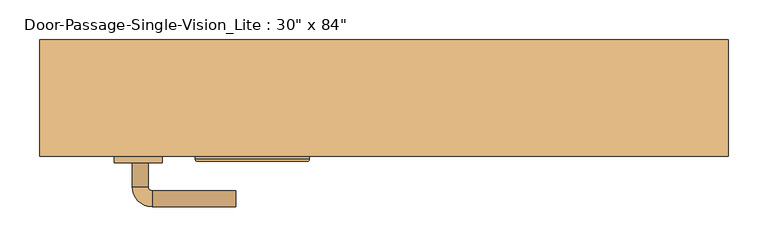
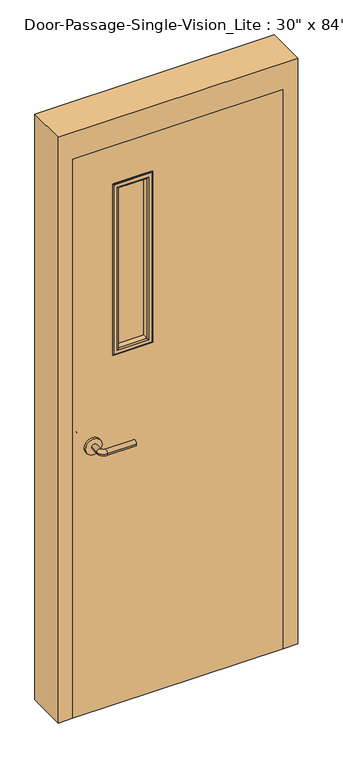
"""IFC4 building model written with IfcOpenShell, lengths in millimetres: door geometry."""

from ifc_helpers import new_model, si_unit, point, frame, frame_2d, origin, place, context, project, spatial, polyline, circle_curve, ellipse_curve, trimmed, segment, composite_curve, outline, extrude, faceted_brep, source, transform, mapped, element, save
from ifc_brep_helpers import plane_surface, cylinder_surface, revolved_surface, advanced_brep


def door_21b9ace8(model_context):
    return source(origin(), model_context, "Body", "SolidModel", [
        advanced_brep(
        [(-315.990625, -4.7, 1016.0), (-295.990625, -4.7, 1016.0), (-315.990625, 25.3, 1016.0), (-295.990625, 25.3, 1016.0), (-290.990625, 30.3, 1016.0), (-290.990625, 50.3, 1016.0), (-185.990625, 50.3, 1016.0), (-185.990625, 30.3, 1016.0)],
        [
            (0, 1, circle_curve(frame((-305.990625, -4.7, 1016.0), z_axis=(0.0, -1.0, 0.0), x_axis=(1.0, 0.0, 0.0)), 10.0)),
            (1, 0, circle_curve(frame((-305.990625, -4.7, 1016.0), z_axis=(0.0, -1.0, 0.0), x_axis=(1.0, 0.0, 0.0)), 10.0)),
            (0, 2),
            (2, 3, circle_curve(frame((-305.990625, 25.3, 1016.0), z_axis=(0.0, -1.0, 0.0), x_axis=(1.0, 0.0, 0.0)), 10.0)),
            (3, 1),
            (3, 2, circle_curve(frame((-305.990625, 25.3, 1016.0), z_axis=(0.0, -1.0, 0.0), x_axis=(1.0, 0.0, 0.0)), 10.0)),
            (4, 3, circle_curve(frame((-290.990625, 25.3, 1016.0), z_axis=(0.0, 0.0, 1.0), x_axis=(-1.0, 0.0, 0.0)), 5.0)),
            (2, 5, circle_curve(frame((-290.990625, 25.3, 1016.0), z_axis=(0.0, 0.0, -1.0), x_axis=(-1.0, 0.0, 0.0)), 25.0)),
            (5, 4, circle_curve(frame((-290.990625, 40.3, 1016.0), z_axis=(-1.0, 0.0, 0.0), x_axis=(0.0, -1.0, 0.0)), 10.0)),
            (4, 5, circle_curve(frame((-290.990625, 40.3, 1016.0), z_axis=(-1.0, 0.0, 0.0), x_axis=(0.0, -1.0, 0.0)), 10.0)),
            (6, 7, circle_curve(frame((-185.990625, 40.3, 1016.0), z_axis=(1.0, 0.0, 0.0), x_axis=(0.0, -1.0, 0.0)), 10.0)),
            (7, 6, circle_curve(frame((-185.990625, 40.3, 1016.0), z_axis=(1.0, 0.0, 0.0), x_axis=(0.0, -1.0, 0.0)), 10.0)),
            (5, 6),
            (7, 4),
        ],
        [
            plane_surface(frame((-305.990625, -4.7, 1016.0), z_axis=(0.0, -1.0, 0.0), x_axis=(0.0, 0.0, 1.0))),
            cylinder_surface(frame((-305.990625, -4.7, 1016.0), z_axis=(0.0, -1.0, 0.0), x_axis=(1.0, 0.0, 0.0)), 10.0),
            revolved_surface(trimmed(ellipse_curve(frame((-305.990625, 25.3, 1016.0), z_axis=(0.0, -1.0, 0.0), x_axis=(1.0, 0.0, 0.0)), 10.0, 10.0), [point((-315.990625, 25.3, 1016.0))], [point((-295.990625, 25.3, 1016.0))], True, "CARTESIAN"), (-290.990625, 25.3, 1016.0), (0.0, 0.0, -1.0)),
            revolved_surface(trimmed(ellipse_curve(frame((-305.990625, 25.3, 1016.0), z_axis=(0.0, -1.0, 0.0), x_axis=(1.0, 0.0, 0.0)), 10.0, 10.0), [point((-295.990625, 25.3, 1016.0))], [point((-315.990625, 25.3, 1016.0))], True, "CARTESIAN"), (-290.990625, 25.3, 1016.0), (0.0, 0.0, -1.0)),
            plane_surface(frame((-185.990625, 40.3, 1016.0), z_axis=(1.0, 0.0, 0.0), x_axis=(0.0, 0.0, 1.0))),
            cylinder_surface(frame((-290.990625, 40.3, 1016.0), z_axis=(-1.0, 0.0, 0.0), x_axis=(0.0, -1.0, 0.0)), 10.0),
        ],
        [
            (0, [[1, 2]]),
            (1, [[-1, 3, 4, 5]]),
            (1, [[-2, -5, 6, -3]]),
            (2, [[7, -4, 8, 9]]),
            (3, [[-8, -6, -7, 10]]),
            (4, [[11, 12]]),
            (5, [[-9, 13, -12, 14]]),
            (5, [[-10, -14, -11, -13]]),
        ],
    ),
        extrude(outline(composite_curve([segment(trimmed(circle_curve(frame_2d((1016.0, -308.490625)), 30.0), [point((1016.0, -338.490625))], [point((1016.0, -278.490625))], False, "CARTESIAN"), True, "CONTINUOUS"), segment(trimmed(circle_curve(frame_2d((1016.0, -308.490625)), 30.0), [point((1016.0, -278.490625))], [point((1016.0, -338.490625))], False, "CARTESIAN"), True, "CONTINUOUS")], self_intersect=False)), frame((0.0, -12.7, 0.0), z_axis=(0.0, 1.0, 0.0), x_axis=(0.0, 0.0, 1.0)), (0.0, 0.0, 1.0), 8.0),
        advanced_brep(
        [(-315.990625, -65.15, 1016.0), (-295.990625, -65.15, 1016.0), (-295.990625, -95.15, 1016.0), (-315.990625, -95.15, 1016.0), (-290.990625, -100.15, 1016.0), (-290.990625, -120.15, 1016.0), (-185.990625, -120.15, 1016.0), (-185.990625, -100.15, 1016.0)],
        [
            (0, 1, circle_curve(frame((-305.990625, -65.15, 1016.0), z_axis=(0.0, 1.0, 0.0), x_axis=(1.0, 0.0, 0.0)), 10.0)),
            (1, 0, circle_curve(frame((-305.990625, -65.15, 1016.0), z_axis=(0.0, 1.0, 0.0), x_axis=(1.0, 0.0, 0.0)), 10.0)),
            (1, 2),
            (2, 3, circle_curve(frame((-305.990625, -95.15, 1016.0), z_axis=(0.0, 1.0, 0.0), x_axis=(1.0, 0.0, 0.0)), 10.0)),
            (3, 0),
            (3, 2, circle_curve(frame((-305.990625, -95.15, 1016.0), z_axis=(0.0, 1.0, 0.0), x_axis=(1.0, 0.0, 0.0)), 10.0)),
            (4, 5, circle_curve(frame((-290.990625, -110.15, 1016.0), z_axis=(-1.0, 0.0, 0.0), x_axis=(0.0, 1.0, 0.0)), 10.0)),
            (5, 3, circle_curve(frame((-290.990625, -95.15, 1016.0), z_axis=(0.0, 0.0, -1.0), x_axis=(-1.0, 0.0, 0.0)), 25.0)),
            (2, 4, circle_curve(frame((-290.990625, -95.15, 1016.0), z_axis=(0.0, 0.0, 1.0), x_axis=(-1.0, 0.0, 0.0)), 5.0)),
            (5, 4, circle_curve(frame((-290.990625, -110.15, 1016.0), z_axis=(-1.0, 0.0, 0.0), x_axis=(0.0, 1.0, 0.0)), 10.0)),
            (6, 7, circle_curve(frame((-185.990625, -110.15, 1016.0), z_axis=(1.0, 0.0, 0.0), x_axis=(0.0, 1.0, 0.0)), 10.0)),
            (7, 6, circle_curve(frame((-185.990625, -110.15, 1016.0), z_axis=(1.0, 0.0, 0.0), x_axis=(0.0, 1.0, 0.0)), 10.0)),
            (4, 7),
            (6, 5),
        ],
        [
            plane_surface(frame((-305.990625, -65.15, 1016.0), z_axis=(0.0, 1.0, 0.0), x_axis=(0.0, 0.0, 1.0))),
            cylinder_surface(frame((-305.990625, -65.15, 1016.0), z_axis=(0.0, 1.0, 0.0), x_axis=(1.0, 0.0, 0.0)), 10.0),
            revolved_surface(trimmed(ellipse_curve(frame((-305.990625, -95.15, 1016.0), z_axis=(0.0, -1.0, 0.0), x_axis=(1.0, 0.0, 0.0)), 10.0, 10.0), [point((-315.990625, -95.15, 1016.0))], [point((-295.990625, -95.15, 1016.0))], True, "CARTESIAN"), (-290.990625, -95.15, 1016.0), (0.0, 0.0, -1.0)),
            revolved_surface(trimmed(ellipse_curve(frame((-305.990625, -95.15, 1016.0), z_axis=(0.0, -1.0, 0.0), x_axis=(1.0, 0.0, 0.0)), 10.0, 10.0), [point((-295.990625, -95.15, 1016.0))], [point((-315.990625, -95.15, 1016.0))], True, "CARTESIAN"), (-290.990625, -95.15, 1016.0), (0.0, 0.0, -1.0)),
            plane_surface(frame((-185.990625, -110.15, 1016.0), z_axis=(1.0, 0.0, 0.0), x_axis=(0.0, 0.0, 1.0))),
            cylinder_surface(frame((-290.990625, -110.15, 1016.0), z_axis=(-1.0, 0.0, 0.0), x_axis=(0.0, 1.0, 0.0)), 10.0),
        ],
        [
            (0, [[1, 2]]),
            (1, [[3, 4, 5, -2]]),
            (1, [[-5, 6, -3, -1]]),
            (2, [[7, 8, -4, 9]]),
            (3, [[10, -9, -6, -8]]),
            (4, [[11, 12]]),
            (5, [[13, -11, 14, -7]]),
            (5, [[-14, -12, -13, -10]]),
        ],
    ),
        extrude(outline(composite_curve([segment(trimmed(circle_curve(frame_2d((1016.0, -308.490625)), 30.0), [point((1016.0, -338.490625))], [point((1016.0, -278.490625))], False, "CARTESIAN"), True, "CONTINUOUS"), segment(trimmed(circle_curve(frame_2d((1016.0, -308.490625)), 30.0), [point((1016.0, -278.490625))], [point((1016.0, -338.490625))], False, "CARTESIAN"), True, "CONTINUOUS")], self_intersect=False)), frame((0.0, -65.15, 0.0), z_axis=(0.0, 1.0, 0.0), x_axis=(0.0, 0.0, 1.0)), (0.0, 0.0, 1.0), 8.0),
        faceted_brep([(381.0, -7.9375, 0.0), (365.125, -7.9375, 0.0), (365.125, 39.6875, 0.0), (381.0, 39.6875, 0.0), (381.0, 88.9, 0.0), (431.8, 88.9, 0.0), (431.8, -57.15, 0.0), (381.0, -57.15, 0.0), (381.0, -57.15, 2133.6), (381.0, -7.9375, 2133.6), (431.8, -57.15, 2235.2), (-431.8, -57.15, 2235.2), (-431.8, -57.15, 0.0), (-381.0, -57.15, 0.0), (-381.0, -57.15, 2133.6), (431.8, 88.9, 2235.2), (381.0, 88.9, 2133.6), (-381.0, 88.9, 2133.6), (-381.0, 88.9, 0.0), (-431.8, 88.9, 0.0), (-431.8, 88.9, 2235.2), (381.0, 39.6875, 2133.6), (365.125, 39.6875, 2117.725), (-365.125, 39.6875, 2117.725), (-365.125, 39.6875, 0.0), (-381.0, 39.6875, 0.0), (-381.0, 39.6875, 2133.6), (365.125, -7.9375, 2117.725), (-381.0, -7.9375, 2133.6), (-381.0, -7.9375, 0.0), (-365.125, -7.9375, 0.0), (-365.125, -7.9375, 2117.725)], [[[0, 1, 2, 3, 4, 5, 6, 7]], [[7, 8, 9, 0]], [[6, 10, 11, 12, 13, 14, 8, 7]], [[5, 15, 10, 6]], [[4, 16, 17, 18, 19, 20, 15, 5]], [[3, 21, 16, 4]], [[2, 22, 23, 24, 25, 26, 21, 3]], [[1, 27, 22, 2]], [[0, 9, 28, 29, 30, 31, 27, 1]], [[8, 14, 28, 9]], [[16, 21, 26, 17]], [[22, 27, 31, 23]], [[12, 19, 18, 25, 24, 30, 29, 13]], [[13, 29, 28, 14]], [[11, 20, 19, 12]], [[17, 26, 25, 18]], [[23, 31, 30, 24]], [[15, 20, 11, 10]]]),
        extrude(outline(polyline([(2133.6, -381.0), (0.0, -381.0), (0.0, 381.0), (2133.6, 381.0), (2133.6, -381.0)]), holes=[polyline([(1981.2, -228.6), (1981.2, -101.6), (1346.2, -101.6), (1346.2, -228.6), (1981.2, -228.6)])]), frame((0.0, -57.15, 0.0), z_axis=(0.0, 1.0, 0.0), x_axis=(0.0, 0.0, 1.0)), (0.0, 0.0, 1.0), 44.45),
        extrude(outline(polyline([(-101.6, -31.75), (-101.6, -38.1), (-228.6, -38.1), (-228.6, -31.75), (-101.6, -31.75)])), frame((0.0, 0.0, 1346.2), z_axis=(0.0, 0.0, 1.0), x_axis=(1.0, 0.0, 0.0)), (0.0, 0.0, 1.0), 635.0),
        advanced_brep(
        [(-228.6, -31.75, 1346.2), (-228.6, -31.75, 1981.2), (-228.6, -12.7, 1981.2), (-228.6, -12.7, 1346.2), (-216.6, -11.7, 1358.2), (-216.6, -11.7, 1969.2), (-216.6, -31.75, 1969.2), (-216.6, -31.75, 1358.2), (-221.6, -6.7, 1353.2), (-221.6, -6.7, 1974.2), (-236.6, -8.7, 1338.2), (-236.6, -8.7, 1989.2), (-234.6, -6.7, 1987.2), (-234.6, -6.7, 1340.2), (-236.6, -12.7, 1338.2), (-236.6, -12.7, 1989.2), (-101.6, -31.75, 1981.2), (-101.6, -12.7, 1981.2), (-113.6, -11.7, 1969.2), (-113.6, -31.75, 1969.2), (-108.6, -6.7, 1974.2), (-93.6, -8.7, 1989.2), (-95.6, -6.7, 1987.2), (-93.6, -12.7, 1989.2), (-101.6, -31.75, 1346.2), (-101.6, -12.7, 1346.2), (-113.6, -11.7, 1358.2), (-113.6, -31.75, 1358.2), (-108.6, -6.7, 1353.2), (-93.6, -8.7, 1338.2), (-95.6, -6.7, 1340.2), (-93.6, -12.7, 1338.2)],
        [
            (0, 1),
            (1, 2),
            (2, 3),
            (3, 0),
            (4, 5),
            (5, 6),
            (6, 7),
            (7, 4),
            (8, 9),
            (9, 5, ellipse_curve(frame((-221.6, -11.7, 1974.2), z_axis=(-0.7071067811865475, 0.0, -0.7071067811865475), x_axis=(0.7071067811865474, 0.0, -0.7071067811865476)), 7.0710678, 5.0)),
            (4, 8, ellipse_curve(frame((-221.6, -11.7, 1353.2), z_axis=(-0.7071067811865475, 0.0, 0.7071067811865475), x_axis=(-0.7071067811865474, 0.0, -0.7071067811865476)), 7.0710678, 5.0)),
            (10, 11),
            (11, 12, ellipse_curve(frame((-234.6, -8.7, 1987.2), z_axis=(-0.7071067811865475, 0.0, -0.7071067811865475), x_axis=(0.7071067811865474, 0.0, -0.7071067811865476)), 2.8284271, 2.0)),
            (12, 13),
            (13, 10, ellipse_curve(frame((-234.6, -8.7, 1340.2), z_axis=(-0.7071067811865475, 0.0, 0.7071067811865475), x_axis=(-0.7071067811865474, 0.0, -0.7071067811865476)), 2.8284271, 2.0)),
            (14, 15),
            (15, 11),
            (10, 14),
            (1, 16),
            (16, 17),
            (17, 2),
            (5, 18),
            (18, 19),
            (19, 6),
            (9, 20),
            (20, 18, ellipse_curve(frame((-108.6, -11.7, 1974.2), z_axis=(-0.7071067811865475, 0.0, 0.7071067811865475), x_axis=(-0.7071067811865476, 0.0, -0.7071067811865474)), 7.0710678, 5.0)),
            (11, 21),
            (21, 22, ellipse_curve(frame((-95.6, -8.7, 1987.2), z_axis=(-0.7071067811865475, 0.0, 0.7071067811865475), x_axis=(-0.7071067811865476, 0.0, -0.7071067811865474)), 2.8284271, 2.0)),
            (22, 12),
            (15, 23),
            (23, 21),
            (16, 24),
            (24, 25),
            (25, 17),
            (18, 26),
            (26, 27),
            (27, 19),
            (20, 28),
            (28, 26, ellipse_curve(frame((-108.6, -11.7, 1353.2), z_axis=(0.7071067811865475, 0.0, 0.7071067811865475), x_axis=(-0.7071067811865474, 0.0, 0.7071067811865476)), 7.0710678, 5.0)),
            (21, 29),
            (29, 30, ellipse_curve(frame((-95.6, -8.7, 1340.2), z_axis=(0.7071067811865475, 0.0, 0.7071067811865475), x_axis=(-0.7071067811865474, 0.0, 0.7071067811865476)), 2.8284271, 2.0)),
            (30, 22),
            (23, 31),
            (31, 29),
            (14, 31),
            (25, 3),
            (24, 0),
            (27, 7),
            (26, 4),
            (28, 8),
            (30, 13),
            (29, 10),
        ],
        [
            plane_surface(frame((-228.6, -12.7, 1346.2), z_axis=(-1.0, 0.0, 0.0), x_axis=(0.0, 0.0, 1.0))),
            plane_surface(frame((-216.6, -31.75, 1358.2), z_axis=(1.0, 0.0, 0.0), x_axis=(0.0, 0.0, 1.0))),
            cylinder_surface(frame((-221.6, -11.7, 1346.2), z_axis=(0.0, 0.0, -1.0), x_axis=(-1.0, 0.0, 0.0)), 5.0),
            cylinder_surface(frame((-234.6, -8.7, 1346.2), z_axis=(0.0, 0.0, -1.0), x_axis=(-1.0, 0.0, 0.0)), 2.0),
            plane_surface(frame((-236.6, -8.7, 1338.2), z_axis=(-1.0, 0.0, 0.0), x_axis=(0.0, 0.0, 1.0))),
            plane_surface(frame((-228.6, -12.7, 1981.2), z_axis=(0.0, 0.0, 1.0), x_axis=(1.0, 0.0, 0.0))),
            plane_surface(frame((-216.6, -31.75, 1969.2), z_axis=(0.0, 0.0, -1.0), x_axis=(1.0, 0.0, 0.0))),
            cylinder_surface(frame((-228.6, -11.7, 1974.2), z_axis=(-1.0, 0.0, 0.0), x_axis=(0.0, 0.0, 1.0)), 5.0),
            cylinder_surface(frame((-228.6, -8.7, 1987.2), z_axis=(-1.0, 0.0, 0.0), x_axis=(0.0, 0.0, 1.0)), 2.0),
            plane_surface(frame((-236.6, -8.7, 1989.2), z_axis=(0.0, 0.0, 1.0), x_axis=(1.0, 0.0, 0.0))),
            plane_surface(frame((-101.6, -12.7, 1981.2), z_axis=(1.0, 0.0, 0.0), x_axis=(0.0, 0.0, -1.0))),
            plane_surface(frame((-113.6, -31.75, 1969.2), z_axis=(-1.0, 0.0, 0.0), x_axis=(0.0, 0.0, -1.0))),
            cylinder_surface(frame((-108.6, -11.7, 1981.2), z_axis=(0.0, 0.0, 1.0), x_axis=(1.0, 0.0, 0.0)), 5.0),
            cylinder_surface(frame((-95.6, -8.7, 1981.2), z_axis=(0.0, 0.0, 1.0), x_axis=(1.0, 0.0, 0.0)), 2.0),
            plane_surface(frame((-93.6, -8.7, 1989.2), z_axis=(1.0, 0.0, 0.0), x_axis=(0.0, 0.0, -1.0))),
            plane_surface(frame((-93.6, -12.7, 1338.2), z_axis=(0.0, -1.0, 0.0), x_axis=(-1.0, 0.0, 0.0))),
            plane_surface(frame((-101.6, -12.7, 1346.2), z_axis=(0.0, 0.0, -1.0), x_axis=(-1.0, 0.0, 0.0))),
            plane_surface(frame((-101.6, -31.75, 1346.2), z_axis=(0.0, -1.0, 0.0), x_axis=(-1.0, 0.0, 0.0))),
            plane_surface(frame((-113.6, -31.75, 1358.2), z_axis=(0.0, 0.0, 1.0), x_axis=(-1.0, 0.0, 0.0))),
            cylinder_surface(frame((-101.6, -11.7, 1353.2), z_axis=(1.0, 0.0, 0.0), x_axis=(0.0, 0.0, -1.0)), 5.0),
            plane_surface(frame((-108.6, -6.7, 1353.2), z_axis=(0.0, 1.0, 0.0), x_axis=(-1.0, 0.0, 0.0))),
            cylinder_surface(frame((-101.6, -8.7, 1340.2), z_axis=(1.0, 0.0, 0.0), x_axis=(0.0, 0.0, -1.0)), 2.0),
            plane_surface(frame((-93.6, -8.7, 1338.2), z_axis=(0.0, 0.0, -1.0), x_axis=(-1.0, 0.0, 0.0))),
        ],
        [
            (0, [[1, 2, 3, 4]]),
            (1, [[5, 6, 7, 8]]),
            (2, [[9, 10, -5, 11]]),
            (3, [[12, 13, 14, 15]]),
            (4, [[16, 17, -12, 18]]),
            (5, [[19, 20, 21, -2]]),
            (6, [[22, 23, 24, -6]]),
            (7, [[25, 26, -22, -10]]),
            (8, [[27, 28, 29, -13]]),
            (9, [[30, 31, -27, -17]]),
            (10, [[32, 33, 34, -20]]),
            (11, [[35, 36, 37, -23]]),
            (12, [[38, 39, -35, -26]]),
            (13, [[40, 41, 42, -28]]),
            (14, [[43, 44, -40, -31]]),
            (15, [[-16, 45, -43, -30], [-3, -21, -34, 46]]),
            (16, [[47, -4, -46, -33]]),
            (17, [[-1, -47, -32, -19], [-7, -24, -37, 48]]),
            (18, [[49, -8, -48, -36]]),
            (19, [[50, -11, -49, -39]]),
            (20, [[-14, -29, -42, 51], [-9, -50, -38, -25]]),
            (21, [[52, -15, -51, -41]]),
            (22, [[-45, -18, -52, -44]]),
        ],
    ),
        advanced_brep(
        [(-228.6, -38.1, 1981.2), (-228.6, -38.1, 1346.2), (-228.6, -57.15, 1346.2), (-228.6, -57.15, 1981.2), (-216.6, -58.15, 1969.2), (-216.6, -58.15, 1358.2), (-216.6, -38.1, 1358.2), (-216.6, -38.1, 1969.2), (-221.6, -63.15, 1974.2), (-221.6, -63.15, 1353.2), (-236.6, -61.15, 1989.2), (-236.6, -61.15, 1338.2), (-234.6, -63.15, 1340.2), (-234.6, -63.15, 1987.2), (-236.6, -57.15, 1989.2), (-236.6, -57.15, 1338.2), (-101.6, -38.1, 1346.2), (-101.6, -57.15, 1346.2), (-113.6, -58.15, 1358.2), (-113.6, -38.1, 1358.2), (-108.6, -63.15, 1353.2), (-93.6, -61.15, 1338.2), (-95.6, -63.15, 1340.2), (-93.6, -57.15, 1338.2), (-101.6, -38.1, 1981.2), (-101.6, -57.15, 1981.2), (-113.6, -58.15, 1969.2), (-113.6, -38.1, 1969.2), (-108.6, -63.15, 1974.2), (-93.6, -61.15, 1989.2), (-95.6, -63.15, 1987.2), (-93.6, -57.15, 1989.2)],
        [
            (0, 1),
            (1, 2),
            (2, 3),
            (3, 0),
            (4, 5),
            (5, 6),
            (6, 7),
            (7, 4),
            (8, 9),
            (9, 5, ellipse_curve(frame((-221.6, -58.15, 1353.2), z_axis=(-0.7071067811865475, 0.0, 0.7071067811865475), x_axis=(0.7071067811865474, 0.0, 0.7071067811865476)), 7.0710678, 5.0)),
            (4, 8, ellipse_curve(frame((-221.6, -58.15, 1974.2), z_axis=(-0.7071067811865475, 0.0, -0.7071067811865475), x_axis=(-0.7071067811865474, 0.0, 0.7071067811865476)), 7.0710678, 5.0)),
            (10, 11),
            (11, 12, ellipse_curve(frame((-234.6, -61.15, 1340.2), z_axis=(-0.7071067811865475, 0.0, 0.7071067811865475), x_axis=(0.7071067811865474, 0.0, 0.7071067811865476)), 2.8284271, 2.0)),
            (12, 13),
            (13, 10, ellipse_curve(frame((-234.6, -61.15, 1987.2), z_axis=(-0.7071067811865475, 0.0, -0.7071067811865475), x_axis=(-0.7071067811865474, 0.0, 0.7071067811865476)), 2.8284271, 2.0)),
            (14, 15),
            (15, 11),
            (10, 14),
            (1, 16),
            (16, 17),
            (17, 2),
            (5, 18),
            (18, 19),
            (19, 6),
            (9, 20),
            (20, 18, ellipse_curve(frame((-108.6, -58.15, 1353.2), z_axis=(-0.7071067811865475, 0.0, -0.7071067811865475), x_axis=(-0.7071067811865476, 0.0, 0.7071067811865474)), 7.0710678, 5.0)),
            (11, 21),
            (21, 22, ellipse_curve(frame((-95.6, -61.15, 1340.2), z_axis=(-0.7071067811865475, 0.0, -0.7071067811865475), x_axis=(-0.7071067811865476, 0.0, 0.7071067811865474)), 2.8284271, 2.0)),
            (22, 12),
            (15, 23),
            (23, 21),
            (16, 24),
            (24, 25),
            (25, 17),
            (18, 26),
            (26, 27),
            (27, 19),
            (20, 28),
            (28, 26, ellipse_curve(frame((-108.6, -58.15, 1974.2), z_axis=(0.7071067811865475, 0.0, -0.7071067811865475), x_axis=(-0.7071067811865474, 0.0, -0.7071067811865476)), 7.0710678, 5.0)),
            (21, 29),
            (29, 30, ellipse_curve(frame((-95.6, -61.15, 1987.2), z_axis=(0.7071067811865475, 0.0, -0.7071067811865475), x_axis=(-0.7071067811865474, 0.0, -0.7071067811865476)), 2.8284271, 2.0)),
            (30, 22),
            (23, 31),
            (31, 29),
            (14, 31),
            (25, 3),
            (24, 0),
            (27, 7),
            (26, 4),
            (28, 8),
            (30, 13),
            (29, 10),
        ],
        [
            plane_surface(frame((-228.6, -57.15, 1981.2), z_axis=(-1.0, 0.0, 0.0), x_axis=(0.0, 0.0, -1.0))),
            plane_surface(frame((-216.6, -38.1, 1969.2), z_axis=(1.0, 0.0, 0.0), x_axis=(0.0, 0.0, -1.0))),
            cylinder_surface(frame((-221.6, -58.15, 1981.2), z_axis=(0.0, 0.0, 1.0), x_axis=(-1.0, 0.0, 0.0)), 5.0),
            cylinder_surface(frame((-234.6, -61.15, 1981.2), z_axis=(0.0, 0.0, 1.0), x_axis=(-1.0, 0.0, 0.0)), 2.0),
            plane_surface(frame((-236.6, -61.15, 1989.2), z_axis=(-1.0, 0.0, 0.0), x_axis=(0.0, 0.0, -1.0))),
            plane_surface(frame((-228.6, -57.15, 1346.2), z_axis=(0.0, 0.0, -1.0), x_axis=(1.0, 0.0, 0.0))),
            plane_surface(frame((-216.6, -38.1, 1358.2), z_axis=(0.0, 0.0, 1.0), x_axis=(1.0, 0.0, 0.0))),
            cylinder_surface(frame((-228.6, -58.15, 1353.2), z_axis=(-1.0, 0.0, 0.0), x_axis=(0.0, 0.0, -1.0)), 5.0),
            cylinder_surface(frame((-228.6, -61.15, 1340.2), z_axis=(-1.0, 0.0, 0.0), x_axis=(0.0, 0.0, -1.0)), 2.0),
            plane_surface(frame((-236.6, -61.15, 1338.2), z_axis=(0.0, 0.0, -1.0), x_axis=(1.0, 0.0, 0.0))),
            plane_surface(frame((-101.6, -57.15, 1346.2), z_axis=(1.0, 0.0, 0.0), x_axis=(0.0, 0.0, 1.0))),
            plane_surface(frame((-113.6, -38.1, 1358.2), z_axis=(-1.0, 0.0, 0.0), x_axis=(0.0, 0.0, 1.0))),
            cylinder_surface(frame((-108.6, -58.15, 1346.2), z_axis=(0.0, 0.0, -1.0), x_axis=(1.0, 0.0, 0.0)), 5.0),
            cylinder_surface(frame((-95.6, -61.15, 1346.2), z_axis=(0.0, 0.0, -1.0), x_axis=(1.0, 0.0, 0.0)), 2.0),
            plane_surface(frame((-93.6, -61.15, 1338.2), z_axis=(1.0, 0.0, 0.0), x_axis=(0.0, 0.0, 1.0))),
            plane_surface(frame((-93.6, -57.15, 1989.2), z_axis=(0.0, 1.0, 0.0), x_axis=(-1.0, 0.0, 0.0))),
            plane_surface(frame((-101.6, -57.15, 1981.2), z_axis=(0.0, 0.0, 1.0), x_axis=(-1.0, 0.0, 0.0))),
            plane_surface(frame((-101.6, -38.1, 1981.2), z_axis=(0.0, 1.0, 0.0), x_axis=(-1.0, 0.0, 0.0))),
            plane_surface(frame((-113.6, -38.1, 1969.2), z_axis=(0.0, 0.0, -1.0), x_axis=(-1.0, 0.0, 0.0))),
            cylinder_surface(frame((-101.6, -58.15, 1974.2), z_axis=(1.0, 0.0, 0.0), x_axis=(0.0, 0.0, 1.0)), 5.0),
            plane_surface(frame((-108.6, -63.15, 1974.2), z_axis=(0.0, -1.0, 0.0), x_axis=(-1.0, 0.0, 0.0))),
            cylinder_surface(frame((-101.6, -61.15, 1987.2), z_axis=(1.0, 0.0, 0.0), x_axis=(0.0, 0.0, 1.0)), 2.0),
            plane_surface(frame((-93.6, -61.15, 1989.2), z_axis=(0.0, 0.0, 1.0), x_axis=(-1.0, 0.0, 0.0))),
        ],
        [
            (0, [[1, 2, 3, 4]]),
            (1, [[5, 6, 7, 8]]),
            (2, [[9, 10, -5, 11]]),
            (3, [[12, 13, 14, 15]]),
            (4, [[16, 17, -12, 18]]),
            (5, [[19, 20, 21, -2]]),
            (6, [[22, 23, 24, -6]]),
            (7, [[25, 26, -22, -10]]),
            (8, [[27, 28, 29, -13]]),
            (9, [[30, 31, -27, -17]]),
            (10, [[32, 33, 34, -20]]),
            (11, [[35, 36, 37, -23]]),
            (12, [[38, 39, -35, -26]]),
            (13, [[40, 41, 42, -28]]),
            (14, [[43, 44, -40, -31]]),
            (15, [[-16, 45, -43, -30], [-3, -21, -34, 46]]),
            (16, [[47, -4, -46, -33]]),
            (17, [[-1, -47, -32, -19], [-7, -24, -37, 48]]),
            (18, [[49, -8, -48, -36]]),
            (19, [[50, -11, -49, -39]]),
            (20, [[-14, -29, -42, 51], [-9, -50, -38, -25]]),
            (21, [[52, -15, -51, -41]]),
            (22, [[-45, -18, -52, -44]]),
        ],
    ),
    ])


if __name__ == "__main__":
    model = new_model("IFC4")
    model_context = context("Model", 3, world=origin())
    ifc_project = project(units=[si_unit("LENGTHUNIT", "METRE", prefix="MILLI")], contexts=[model_context])
    site = spatial("IfcSite", under=ifc_project)
    building = spatial("IfcBuilding", under=site)
    placement = place(None, origin())
    door_shape = door_21b9ace8(model_context)
    element("IfcDoor", 1, ObjectType="Door-Passage-Single-Vision_Lite : 30\" x 84\"", at=placement, inside=building, context=model_context, shape_type="MappedRepresentation", body=[
        mapped(door_shape, transform((0.0, 0.0, 0.0), x_axis=(1.0, 0.0, 0.0), y_axis=(0.0, 1.0, 0.0), z_axis=(0.0, 0.0, 1.0))),
    ])
    save(model, "model.ifc")

# Revit data of these elements
# Type "Door-Passage-Single-Vision_Lite : 30\" x 84\""
#   Type Mark = "20"
#   Assembly Code = "B2030100"
#   Analytic Construction = "Wooden"
#   Thickness = 0' - 1 3/4"
#   Thermal Resistance (R) = 2.5876 (h·ft²·°F)/BTU
#   Swing Angle [instance default] = 90.00°
#   Strike Height = 3' - 4"
#   Rough Width [instance default] = 2' - 10"
#   Rough Height [instance default] = 7' - 4"
#   MFOpeningHeight [instance default] = 0' - 4"
#   MFOpeningWidth [instance default] = 0' - 4"
#   Inset Calculate [instance default] = 0' - 4"
#   Masonry Inset [instance default] = 0' - 1"
#   Height = 7' - 0"
#   Width = 2' - 6"
#   Heat Transfer Coefficient (U) = 0.3865 BTU/(h·ft²·°F)
#   Masonry Frame Depth = 0' - 5 3/4"
#   Masonry Frame [instance default] = yes
#   Function = 1
#   Dry Wall Frame [instance default] = no
#   Define Thermal Properties by = 1
#   Panel Material = Wood - Birch
#   Glazing = Glass
#   Glass Stop Material = Metal - Paint Finish - Grey
#   Frame Material = Metal - Paint Finish - Grey
#   Door Handle Material = Aluminum
#   Visual Light Transmittance = 0
#   Solar Heat Gain Coefficient = 0
#   Wall Closure = (empty or 0)
# Element 1 (IfcDoor, "Door-Passage-Single-Vision_Lite : 30\" x 84\"")
#   Materials on its faces: "Metal - Paint Finish - Grey", "Aluminum", "Wood - Birch", "Glass"
# Materials
#   "Wood - Birch": class "Wood", colour RGB 173 132 96, transparency 0, Cost = 0
#   "Glass": class "Glass", colour RGB 245 245 243, transparency 1, Description = "Soda Lime Glass", Cost = 0
#   "Metal - Paint Finish - Grey": class "Paint", colour RGB 178 178 178, transparency 0, Cost = 0
#   "Aluminum": class "Metal", colour RGB 244 245 246, transparency 0, Description = "Aluminum 6061", Cost = 0
